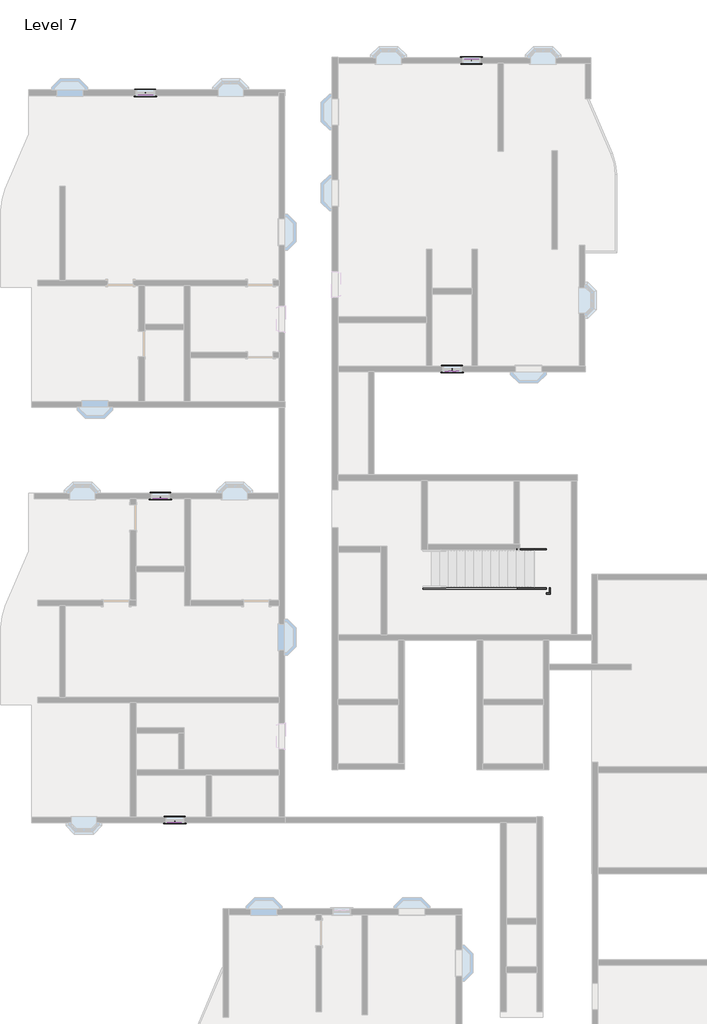
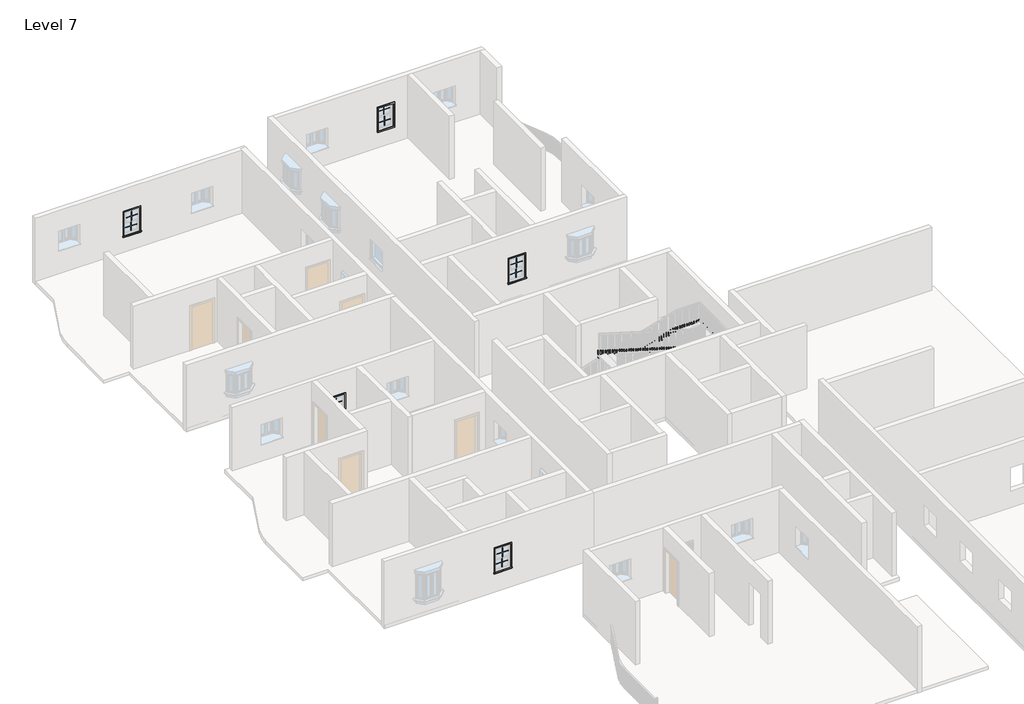
# One storey, part 14 of 14: 20 proxies, 6 members.
"""IFC4 building model written with IfcOpenShell, lengths in millimetres."""

from ifc_helpers import new_model, si_unit, frame, origin, place, context, project, spatial, polyline, outline, extrude, transform, mapped, element, save
from components import muntin_pattern_2x2_muntin_pattern_2x2_c35c595f, trim_window_exterior_flat_with_sill_e38017c9, trim_window_interior_flat_picture_frame_d728ed12

model = new_model("IFC4")

# Units and contexts
model_context = context("Model", 3, world=origin())
ifc_project = project(units=[si_unit("LENGTHUNIT", "METRE", prefix="MILLI")], contexts=[model_context])

# Site, building, storey
site = spatial("IfcSite", under=ifc_project)
building = spatial("IfcBuilding", under=site)
storey = spatial("IfcBuildingStorey", under=building, Name="Level 7", Elevation=18288.0)

# Proxies
placement = place(None, origin())
muntin_pattern_2x2_muntin_pattern_2x2_shape = muntin_pattern_2x2_muntin_pattern_2x2_c35c595f(model_context)
element("IfcBuildingElementProxy", 1, Name="Muntin Pattern_2x2 : Muntin Pattern_2x2", ObjectType="Muntin Pattern_2x2 : Muntin Pattern_2x2", at=placement, inside=storey, context=model_context, shape_type="MappedRepresentation", body=[
    mapped(muntin_pattern_2x2_muntin_pattern_2x2_shape, transform((-14639.3891351, 14368.0833494, 19758.025), x_axis=(-1.0, 0.0, 0.0), y_axis=(0.0, -1.0, 0.0), z_axis=(0.0, 0.0, 1.0))),
])
element("IfcBuildingElementProxy", 2, Name="Muntin Pattern_2x2 : Muntin Pattern_2x2", ObjectType="Muntin Pattern_2x2 : Muntin Pattern_2x2", at=placement, inside=storey, context=model_context, shape_type="MappedRepresentation", body=[
    mapped(muntin_pattern_2x2_muntin_pattern_2x2_shape, transform((-14639.3891351, 14412.5333494, 19278.6), x_axis=(-1.0, 0.0, 0.0), y_axis=(0.0, -1.0, 0.0), z_axis=(0.0, 0.0, 1.0))),
])
element("IfcBuildingElementProxy", 3, Name="Muntin Pattern_2x2 : Muntin Pattern_2x2", ObjectType="Muntin Pattern_2x2 : Muntin Pattern_2x2", at=placement, inside=storey, context=model_context, shape_type="MappedRepresentation", body=[
    mapped(muntin_pattern_2x2_muntin_pattern_2x2_shape, transform((-14125.0391351, 2785.6833494, 19758.025), x_axis=(-1.0, 0.0, 0.0), y_axis=(0.0, -1.0, 0.0), z_axis=(0.0, 0.0, 1.0))),
])
element("IfcBuildingElementProxy", 4, Name="Muntin Pattern_2x2 : Muntin Pattern_2x2", ObjectType="Muntin Pattern_2x2 : Muntin Pattern_2x2", at=placement, inside=storey, context=model_context, shape_type="MappedRepresentation", body=[
    mapped(muntin_pattern_2x2_muntin_pattern_2x2_shape, transform((-14125.0391351, 2830.1333494, 19278.6), x_axis=(-1.0, 0.0, 0.0), y_axis=(0.0, -1.0, 0.0), z_axis=(0.0, 0.0, 1.0))),
])
element("IfcBuildingElementProxy", 5, Name="Muntin Pattern_2x2 : Muntin Pattern_2x2", ObjectType="Muntin Pattern_2x2 : Muntin Pattern_2x2", at=placement, inside=storey, context=model_context, shape_type="MappedRepresentation", body=[
    mapped(muntin_pattern_2x2_muntin_pattern_2x2_shape, transform((-4206.3391351, 18910.0465905, 19758.025), x_axis=(-1.0, 0.0, 0.0), y_axis=(0.0, -1.0, 0.0), z_axis=(0.0, 0.0, 1.0))),
])
element("IfcBuildingElementProxy", 6, Name="Muntin Pattern_2x2 : Muntin Pattern_2x2", ObjectType="Muntin Pattern_2x2 : Muntin Pattern_2x2", at=placement, inside=storey, context=model_context, shape_type="MappedRepresentation", body=[
    mapped(muntin_pattern_2x2_muntin_pattern_2x2_shape, transform((-4206.3391351, 18954.4965905, 19278.6), x_axis=(-1.0, 0.0, 0.0), y_axis=(0.0, -1.0, 0.0), z_axis=(0.0, 0.0, 1.0))),
])
element("IfcBuildingElementProxy", 7, Name="Muntin Pattern_2x2 : Muntin Pattern_2x2", ObjectType="Muntin Pattern_2x2 : Muntin Pattern_2x2", at=placement, inside=storey, context=model_context, shape_type="MappedRepresentation", body=[
    mapped(muntin_pattern_2x2_muntin_pattern_2x2_shape, transform((-3514.1891351, 30066.9965905, 19758.025), x_axis=(1.0, 0.0, 0.0), y_axis=(0.0, 1.0, 0.0), z_axis=(0.0, 0.0, 1.0))),
])
element("IfcBuildingElementProxy", 8, Name="Muntin Pattern_2x2 : Muntin Pattern_2x2", ObjectType="Muntin Pattern_2x2 : Muntin Pattern_2x2", at=placement, inside=storey, context=model_context, shape_type="MappedRepresentation", body=[
    mapped(muntin_pattern_2x2_muntin_pattern_2x2_shape, transform((-3514.1891351, 30022.5465905, 19278.6), x_axis=(1.0, 0.0, 0.0), y_axis=(0.0, 1.0, 0.0), z_axis=(0.0, 0.0, 1.0))),
])
element("IfcBuildingElementProxy", 9, Name="Muntin Pattern_2x2 : Muntin Pattern_2x2", ObjectType="Muntin Pattern_2x2 : Muntin Pattern_2x2", at=placement, inside=storey, context=model_context, shape_type="MappedRepresentation", body=[
    mapped(muntin_pattern_2x2_muntin_pattern_2x2_shape, transform((-15175.9641351, 28782.5833494, 19758.025), x_axis=(-1.0, 0.0, 0.0), y_axis=(0.0, -1.0, 0.0), z_axis=(0.0, 0.0, 1.0))),
])
element("IfcBuildingElementProxy", 10, Name="Muntin Pattern_2x2 : Muntin Pattern_2x2", ObjectType="Muntin Pattern_2x2 : Muntin Pattern_2x2", at=placement, inside=storey, context=model_context, shape_type="MappedRepresentation", body=[
    mapped(muntin_pattern_2x2_muntin_pattern_2x2_shape, transform((-15175.9641351, 28827.0333494, 19278.6), x_axis=(-1.0, 0.0, 0.0), y_axis=(0.0, -1.0, 0.0), z_axis=(0.0, 0.0, 1.0))),
])
trim_window_exterior_flat_with_sill_shape = trim_window_exterior_flat_with_sill_e38017c9(model_context)
element("IfcBuildingElementProxy", 11, Name="Trim-Window-Exterior-Flat : with Sill", ObjectType="Trim-Window-Exterior-Flat : with Sill", at=placement, inside=storey, context=model_context, shape_type="MappedRepresentation", body=[
    mapped(trim_window_exterior_flat_with_sill_shape, transform((-14639.3891351, 14333.1583494, 20269.2), x_axis=(1.0, 0.0, 0.0), y_axis=(0.0, 0.0, 1.0), z_axis=(0.0, -1.0, 0.0))),
])
element("IfcBuildingElementProxy", 12, Name="Trim-Window-Exterior-Flat : with Sill", ObjectType="Trim-Window-Exterior-Flat : with Sill", at=placement, inside=storey, context=model_context, shape_type="MappedRepresentation", body=[
    mapped(trim_window_exterior_flat_with_sill_shape, transform((-14125.0391351, 2750.7583494, 20269.2), x_axis=(1.0, 0.0, 0.0), y_axis=(0.0, 0.0, 1.0), z_axis=(0.0, -1.0, 0.0))),
])
element("IfcBuildingElementProxy", 13, Name="Trim-Window-Exterior-Flat : with Sill", ObjectType="Trim-Window-Exterior-Flat : with Sill", at=placement, inside=storey, context=model_context, shape_type="MappedRepresentation", body=[
    mapped(trim_window_exterior_flat_with_sill_shape, transform((-4206.3391351, 18875.1215905, 20269.2), x_axis=(1.0, 0.0, 0.0), y_axis=(0.0, 0.0, 1.0), z_axis=(0.0, -1.0, 0.0))),
])
element("IfcBuildingElementProxy", 14, Name="Trim-Window-Exterior-Flat : with Sill", ObjectType="Trim-Window-Exterior-Flat : with Sill", at=placement, inside=storey, context=model_context, shape_type="MappedRepresentation", body=[
    mapped(trim_window_exterior_flat_with_sill_shape, transform((-3514.1891351, 30101.9215905, 20269.2), x_axis=(-1.0, 0.0, 0.0), y_axis=(0.0, 0.0, 1.0), z_axis=(0.0, 1.0, 0.0))),
])
element("IfcBuildingElementProxy", 15, Name="Trim-Window-Exterior-Flat : with Sill", ObjectType="Trim-Window-Exterior-Flat : with Sill", at=placement, inside=storey, context=model_context, shape_type="MappedRepresentation", body=[
    mapped(trim_window_exterior_flat_with_sill_shape, transform((-15175.9641351, 28747.6583494, 20269.2), x_axis=(1.0, 0.0, 0.0), y_axis=(0.0, 0.0, 1.0), z_axis=(0.0, -1.0, 0.0))),
])
trim_window_interior_flat_picture_frame_shape = trim_window_interior_flat_picture_frame_d728ed12(model_context)
element("IfcBuildingElementProxy", 16, Name="Trim-Window-Interior-Flat : Picture Frame", ObjectType="Trim-Window-Interior-Flat : Picture Frame", at=placement, inside=storey, context=model_context, shape_type="MappedRepresentation", body=[
    mapped(trim_window_interior_flat_picture_frame_shape, transform((-14639.3891351, 14536.3583494, 20269.2), x_axis=(-1.0, 0.0, 0.0), y_axis=(0.0, 0.0, 1.0), z_axis=(0.0, 1.0, 0.0))),
])
element("IfcBuildingElementProxy", 17, Name="Trim-Window-Interior-Flat : Picture Frame", ObjectType="Trim-Window-Interior-Flat : Picture Frame", at=placement, inside=storey, context=model_context, shape_type="MappedRepresentation", body=[
    mapped(trim_window_interior_flat_picture_frame_shape, transform((-14125.0391351, 2953.9583494, 20269.2), x_axis=(-1.0, 0.0, 0.0), y_axis=(0.0, 0.0, 1.0), z_axis=(0.0, 1.0, 0.0))),
])
element("IfcBuildingElementProxy", 18, Name="Trim-Window-Interior-Flat : Picture Frame", ObjectType="Trim-Window-Interior-Flat : Picture Frame", at=placement, inside=storey, context=model_context, shape_type="MappedRepresentation", body=[
    mapped(trim_window_interior_flat_picture_frame_shape, transform((-4206.3391351, 19078.3215905, 20269.2), x_axis=(-1.0, 0.0, 0.0), y_axis=(0.0, 0.0, 1.0), z_axis=(0.0, 1.0, 0.0))),
])
element("IfcBuildingElementProxy", 19, Name="Trim-Window-Interior-Flat : Picture Frame", ObjectType="Trim-Window-Interior-Flat : Picture Frame", at=placement, inside=storey, context=model_context, shape_type="MappedRepresentation", body=[
    mapped(trim_window_interior_flat_picture_frame_shape, transform((-3514.1891351, 29898.7215905, 20269.2), x_axis=(1.0, 0.0, 0.0), y_axis=(0.0, 0.0, 1.0), z_axis=(0.0, -1.0, 0.0))),
])
element("IfcBuildingElementProxy", 20, Name="Trim-Window-Interior-Flat : Picture Frame", ObjectType="Trim-Window-Interior-Flat : Picture Frame", at=placement, inside=storey, context=model_context, shape_type="MappedRepresentation", body=[
    mapped(trim_window_interior_flat_picture_frame_shape, transform((-15175.9641351, 28950.8583494, 20269.2), x_axis=(-1.0, 0.0, 0.0), y_axis=(0.0, 0.0, 1.0), z_axis=(0.0, 1.0, 0.0))),
])

# Members
element("IfcMember", 21, ObjectType="Stringer - 2\" Width", at=placement, inside=storey, context=model_context, shape_type="SweptSolid", body=[
    extrude(outline(polyline([(18479.5995961, -5254.0891351), (18288.0, -5254.0891351), (18288.0, -4832.019314), (19735.8, -6.019314), (19735.8, -1066.7544553), (18479.5995961, -5254.0891351)])), frame((0.0, 12506.0715905, 0.0), z_axis=(0.0, 1.0, 0.0), x_axis=(0.0, 0.0, 1.0)), (0.0, 0.0, 1.0), 50.8),
])
element("IfcMember", 22, ObjectType="Stringer - 2\" Width", at=placement, inside=storey, context=model_context, shape_type="SweptSolid", body=[
    extrude(outline(polyline([(54.5108649, 12556.8715905), (105.3108649, 12556.8715905), (105.3108649, 9478.4949943), (54.5108649, 9478.4949943), (54.5108649, 12556.8715905)])), frame((0.0, 0.0, 19431.0), z_axis=(0.0, 0.0, 1.0), x_axis=(1.0, 0.0, 0.0)), (0.0, 0.0, 1.0), 304.8),
])
element("IfcMember", 23, ObjectType="Stringer - 2\" Width", at=placement, inside=storey, context=model_context, shape_type="SweptSolid", body=[
    extrude(outline(polyline([(19431.0, 105.3108649), (19523.5395961, 105.3108649), (21131.3595961, -5254.0891351), (20813.1390537, -5254.0891351), (19431.0, -646.9589562), (19431.0, 105.3108649)])), frame((0.0, 9427.6949943, 0.0), z_axis=(0.0, 1.0, 0.0), x_axis=(0.0, 0.0, 1.0)), (0.0, 0.0, 1.0), 50.8),
])
element("IfcMember", 24, ObjectType="Stringer - 2\" Width", at=placement, inside=storey, context=model_context, shape_type="SweptSolid", body=[
    extrude(outline(polyline([(18479.5995961, -5254.0891351), (18288.0, -5254.0891351), (18288.0, -4832.019314), (19517.7390537, -732.8891351), (19735.8, -732.8891351), (19735.8, -1066.7544553), (18479.5995961, -5254.0891351)])), frame((0.0, 11103.4082924, 0.0), z_axis=(0.0, 1.0, 0.0), x_axis=(0.0, 0.0, 1.0)), (0.0, 0.0, 1.0), 50.8),
])
element("IfcMember", 25, ObjectType="Stringer - 2\" Width", at=placement, inside=storey, context=model_context, shape_type="SweptSolid", body=[
    extrude(outline(polyline([(-732.8891351, 11154.2082924), (-682.0891351, 11154.2082924), (-682.0891351, 10976.4082924), (-732.8891351, 10976.4082924), (-732.8891351, 11154.2082924)])), frame((0.0, 0.0, 19431.0), z_axis=(0.0, 0.0, 1.0), x_axis=(1.0, 0.0, 0.0)), (0.0, 0.0, 1.0), 304.8),
])
element("IfcMember", 26, ObjectType="Stringer - 2\" Width", at=placement, inside=storey, context=model_context, shape_type="SweptSolid", body=[
    extrude(outline(polyline([(19441.5390537, -682.0891351), (19759.7595961, -682.0891351), (21131.3595961, -5254.0891351), (20813.1390537, -5254.0891351), (19441.5390537, -682.0891351)])), frame((0.0, 10925.6082924, 0.0), z_axis=(0.0, 1.0, 0.0), x_axis=(0.0, 0.0, 1.0)), (0.0, 0.0, 1.0), 50.8),
])

save(model, "model.ifc")

# Revit data of these elements
# Type "Muntin Pattern_2x2 : Muntin Pattern_2x2"
#   Width [instance default] = 4' - 0"
#   Thickness = 0' - 0 1/2"
#   Height [instance default] = 4' - 0"
#   Distance = 0' - 0 3/4"
#   Interior Material [instance default] = none
#   Exterior Material [instance default] = none
#   Default Elevation = 0
# Type "Trim-Window-Exterior-Flat : with Sill"
#   Trim Width = 0' - 2 1/4"
#   Trim Thickness_Picture Frame = 0' - 1 1/4"
#   Trim Thickness_with Sill = 0' - 0 3/4"
#   Sill Thickness = 0' - 1 1/4"
#   Opening Width [instance default] = 2' - 0"
#   Opening Height [instance default] = 3' - 0"
#   Default Elevation = 4' - 0"
#   Sill = yes
#   Picture Frame = no
#   Trim Material [instance default] = none
# Type "Trim-Window-Interior-Flat : Picture Frame"
#   Trim Thickness_Picture Frame = 0' - 1 1/4"
#   Trim Width = 0' - 2 1/4"
#   Trim Thickness_with Sill = 0' - 0 3/4"
#   Sill Thickness = 0' - 1 1/4"
#   Opening Width [instance default] = 2' - 0"
#   Opening Height [instance default] = 3' - 0"
#   Default Elevation = 4' - 0"
#   Sill = no
#   Picture Frame = yes
#   Trim Material [instance default] = none
# Elements 1, 2, 3, 4, 5, 6, 7, 8, 9, 10 (IfcBuildingElementProxy, "Muntin Pattern_2x2 : Muntin Pattern_2x2")
#   Width = 1' - 8"
#   Height = 1' - 5 1/8"
#   Interior Material = Wood - Stained
#   Exterior Material = Clad - White
#   Phase Created = New Construction
#   Materials on its faces: "Clad - White", "Wood - Stained"
# Elements 11, 12, 13, 14, 15 (IfcBuildingElementProxy, "Trim-Window-Exterior-Flat : with Sill")
#   Opening Width = 2' - 2"
#   Opening Height = 3' - 6"
#   Trim Material = Clad - White
#   Phase Created = New Construction
#   Materials on its faces: "Clad - White"
# Elements 16, 17, 18, 19, 20 (IfcBuildingElementProxy, "Trim-Window-Interior-Flat : Picture Frame")
#   Opening Width = 2' - 2"
#   Opening Height = 3' - 6"
#   Trim Material = Wood - Stained
#   Phase Created = New Construction
#   Materials on its faces: "Wood - Stained"
# Elements 21, 22, 23, 24, 25, 26 (IfcMember, "Stringer - 2\" Width")
#   Phase Created = New Construction
# Materials
#   "Clad - White": class "Wood", colour RGB 242 242 238, transparency 0, Cost = 0
#   "Wood - Stained": class "Wood", colour RGB 224 178 126, transparency 0, Cost = 0
